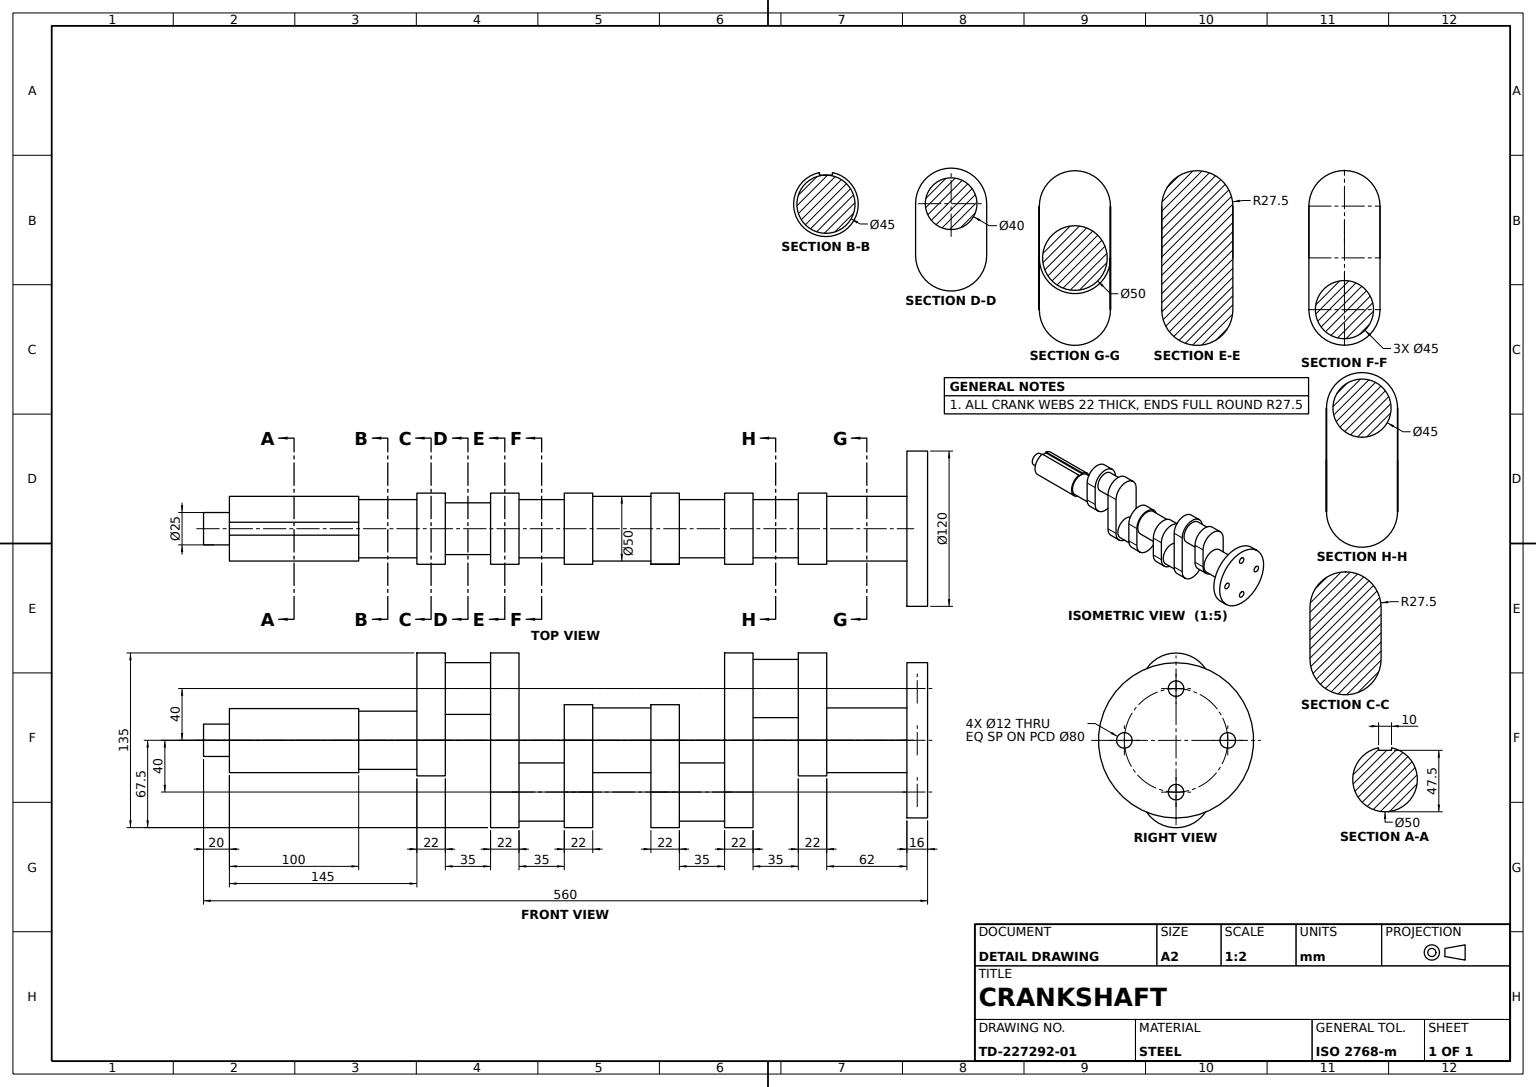
SolidWorks part; units mm, degrees
material "Plain Carbon Steel"
ref_plane "Front Plane" through (0, 0, 0) normal (0, 0, 1) x (1, 0, 0)
ref_plane "Top Plane" through (0, 0, 0) normal (0, 1, 0) x (1, 0, 0)
ref_plane "Right Plane" through (0, 0, 0) normal (1, 0, 0) x (0, 0, -1)
sketch "Flange Sketch" plane through (0, 0, 0) normal (0, 0, 1) x (1, 0, 0)
  line L0 (-383.9492, 0) -> (402.1315, 0) construction
  line L2 (0, 213.0357) -> (0, -254.2489) construction
  circle A0 centre (0, 0) radius 60
  dimension "D1" = 120
extrude "Flange Ø120x16" add sketch "Flange Sketch" along normal blind 16
sketch "Front Shaft Sketch" plane through (0, 0, 16) normal (0, 0, 1) x (1, 0, 0)
  circle A0 centre (0, 0) radius 25
  dimension "D1" = 50
extrude "Front Shaft Ø50x62" add sketch "Front Shaft Sketch" along normal blind 62
sketch "Crank Web 1 Sketch" plane through (0, 0, 78) normal (0, 0, 1) x (1, 0, 0)
  line L0 (0, 0) -> (-40, 0) construction
  line L1 (0, -27.5) -> (-40, -27.5)
  line L2 (0, 27.5) -> (-40, 27.5)
  arc A0 (0, -27.5) -> (0, 27.5) centre (0, 0) ccw
  arc A1 (-40, 27.5) -> (-40, -27.5) centre (-40, 0) ccw
  point P3 (-20, 0)
  dimension "D1" = 27.5
  dimension "D2" = 40
extrude "Crank Web 1" add sketch "Crank Web 1 Sketch" along normal blind 22
sketch "Crankpin 1 Sketch" plane through (0, 0, 100) normal (0, 0, 1) x (1, 0, 0)
  circle A0 centre (-40, 0) radius 22.5
  dimension "D1" = 45
extrude "Crankpin 1 Ø45" add sketch "Crankpin 1 Sketch" along normal blind 35
sketch "Crank Web 2 Sketch" plane through (0, 0, 135) normal (0, 0, 1) x (1, 0, 0)
  line L0 (-40, 0) -> (40, 0) construction
  line L1 (-40, 27.5) -> (40, 27.5)
  line L2 (-40, -27.5) -> (40, -27.5)
  arc A0 (-40, 27.5) -> (-40, -27.5) centre (-40, 0) ccw
  arc A1 (40, -27.5) -> (40, 27.5) centre (40, 0) ccw
  point P4 (0, 0)
  dimension "D2" = 27.5
  dimension "D1" = 80
extrude "Crank Web 2" add sketch "Crank Web 2 Sketch" along normal blind 22
sketch "Crankpin 2 Sketch" plane through (0, 0, 157) normal (0, 0, 1) x (1, 0, 0)
  circle A0 centre (40, 0) radius 22.5
  dimension "D1" = 45
extrude "Crankpin 2 Ø45" add sketch "Crankpin 2 Sketch" along normal blind 35
sketch "Crank Web 3 Sketch" plane through (0, 0, 192) normal (0, 0, 1) x (1, 0, 0)
  line L0 (40, 0) -> (0, 0) construction
  line L1 (40, -27.5) -> (0, -27.5)
  line L2 (40, 27.5) -> (0, 27.5)
  arc A0 (40, -27.5) -> (40, 27.5) centre (40, 0) ccw
  arc A1 (0, 27.5) -> (0, -27.5) centre (0, 0) ccw
  point P4 (20, 0)
  dimension "D2" = 27.5
  dimension "D1" = 40
extrude "Crank Web 3" add sketch "Crank Web 3 Sketch" along normal blind 22
sketch "Centre Main Journal Sketch" plane through (0, 0, 214) normal (0, 0, 1) x (1, 0, 0)
  circle A0 centre (0, 0) radius 25
  dimension "D1" = 50
extrude "Centre Main Journal Ø50" add sketch "Centre Main Journal Sketch" along normal blind 45
sketch "Crank Web 4 Sketch" plane through (0, 0, 259) normal (0, 0, 1) x (1, 0, 0)
  line L0 (0, 0) -> (40, 0) construction
  line L1 (0, 27.5) -> (40, 27.5)
  line L2 (0, -27.5) -> (40, -27.5)
  arc A0 (0, 27.5) -> (0, -27.5) centre (0, 0) ccw
  arc A1 (40, -27.5) -> (40, 27.5) centre (40, 0) ccw
  point P3 (20, 0)
  dimension "D2" = 27.5
  dimension "D1" = 40
extrude "Crank Web 4" add sketch "Crank Web 4 Sketch" along normal blind 22
sketch "Crankpin 3 Sketch" plane through (0, 0, 281) normal (0, 0, 1) x (1, 0, 0)
  circle A0 centre (40, 0) radius 22.5
  dimension "D1" = 45
extrude "Crankpin 3 Ø45" add sketch "Crankpin 3 Sketch" along normal blind 35
sketch "Crank Web 5 Sketch" plane through (0, 0, 316) normal (0, 0, 1) x (1, 0, 0)
  line L0 (40, 0) -> (-40, 0) construction
  line L1 (40, -27.5) -> (-40, -27.5)
  line L2 (40, 27.5) -> (-40, 27.5)
  arc A0 (40, -27.5) -> (40, 27.5) centre (40, 0) ccw
  arc A1 (-40, 27.5) -> (-40, -27.5) centre (-40, 0) ccw
  point P4 (0, 0)
  dimension "D2" = 27.5
  dimension "D1" = 80
extrude "Crank Web 5" add sketch "Crank Web 5 Sketch" along normal blind 22
sketch "Crankpin 4 Sketch" plane through (0, 0, 338) normal (0, 0, 1) x (1, 0, 0)
  circle A0 centre (-40, 0) radius 20
  dimension "D1" = 40
extrude "Crankpin 4 Ø40" add sketch "Crankpin 4 Sketch" along normal blind 35
sketch "Crank Web 6 Sketch" plane through (0, 0, 373) normal (0, 0, 1) x (1, 0, 0)
  line L0 (-40, 0) -> (0, 0) construction
  line L1 (-40, 27.5) -> (0, 27.5)
  line L2 (-40, -27.5) -> (0, -27.5)
  arc A0 (-40, 27.5) -> (-40, -27.5) centre (-40, 0) ccw
  arc A1 (0, -27.5) -> (0, 27.5) centre (0, 0) ccw
  point P4 (-20, 0)
  dimension "D2" = 27.5
  dimension "D1" = 40
extrude "Crank Web 6" add sketch "Crank Web 6 Sketch" along normal blind 22
sketch "Rear Shaft Sketch" plane through (0, 0, 395) normal (0, 0, 1) x (1, 0, 0)
  circle A0 centre (0, 0) radius 22.5
  dimension "D1" = 45
extrude "Rear Shaft Ø45x145" add sketch "Rear Shaft Sketch" along normal blind 145
sketch "Rear Shaft Step Sketch" plane through (0, 0, 540) normal (0, 0, 1) x (1, 0, 0)
  circle A0 centre (0, 0) radius 25
  dimension "D1" = 50
extrude "Rear Shaft Step Ø50x100" add sketch "Rear Shaft Step Sketch" against normal blind 100
sketch "Rear Shaft Cut Sketch" plane through (0, 0, 540) normal (0, 0, 1) x (1, 0, 0)
  line L0 (-116.663, 0) -> (103.4233, 0) construction
  line L1 (0, 72.6787) -> (0, -77.6193) construction
  line L3 (-24.4949, -5) -> (-22.5, -5)
  line L5 (-24.4949, 5) -> (-22.5, 5)
  line L6 (-22.5, -5) -> (-22.5, 5)
  line L7 (-25, 0) -> (-22.5, 5) construction
  line L8 (-25, 0) -> (-22.5, -5) construction
  circle A0 centre (0, 0) radius 25 construction
  circle A1 centre (0, 0) radius 25 construction
  circle A2 centre (0, 0) radius 25
  arc A3 (-24.4949, 5) -> (-24.4949, -5) centre (0, 0) ccw
  point P5 (-25, 0)
  dimension "D1" = 22.5
  dimension "D2" = 24.4949
  dimension "D3" = 0
extrude "Rear Shaft Profile Cut" cut sketch "Rear Shaft Cut Sketch" against normal blind 100
sketch "End Stub Sketch" plane through (0, 0, 540) normal (0, 0, 1) x (1, 0, 0)
  circle A0 centre (0, 0) radius 12.5
  dimension "D1" = 25
extrude "End Stub Ø25x20" add sketch "End Stub Sketch" along normal blind 20
sketch "Flange Bolt Holes Sketch" plane through (0, 0, 16) normal (0, 0, 1) x (1, 0, 0)
  line L0 (-154.1827, 0) -> (192.3618, 0) construction
  line L1 (0, 92.1099) -> (0, -101.9173) construction
  circle A0 centre (0, 40) radius 6
  circle A1 centre (0, -40) radius 6
  circle A2 centre (-40, 0) radius 6
  circle A3 centre (40, 0) radius 6
  dimension "D1" = 12
  dimension "D2" = 40
  dimension "D3" = 12
  dimension "D5" = 12
  dimension "D6" = 40
  dimension "D7" = 12
  dimension "D4" = 40
  dimension "D8" = 40
extrude "Flange Bolt Holes 4xØ12" cut sketch "Flange Bolt Holes Sketch" against normal blind 20
